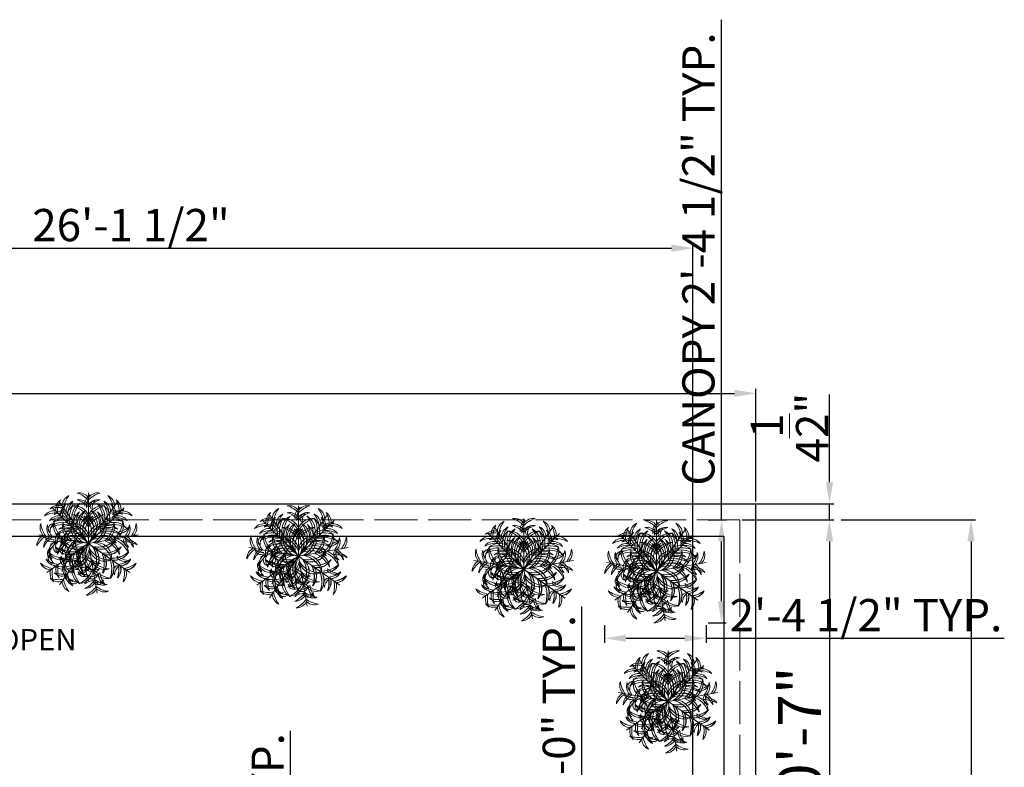
# Model space of a CAD drawing. Units: millimetres. Extents: x 595116 to 630915, y 909473 to 920225.
# Tile 126 of 134: x 629637 to 629912, y 920016 to 920225. Entities that reach past the tile are written whole.
import ezdxf

# ---------------------------------------------------------------- set-up
doc = ezdxf.new("R2010")
doc.units = ezdxf.units.MM
doc.linetypes.add('ACAD_ISO02W100', pattern=[15, 12, -3])
for name, color, linetype, lineweight in [('A-AREA-IDEN', 7, 'Continuous', 20), ('C-PROP', 7, 'Continuous', 25), ('C-PROP-REF', 240, 'ACAD_ISO02W100', 13), ('Dimension', 3, 'Continuous', 18), ('L-PLNT', 85, 'Continuous', 13)]:
    doc.layers.add(name, color=color, linetype=linetype, lineweight=lineweight)
doc.styles.get("Standard").update_dxf_attribs({"font": 'arial.ttf'})
doc.dimstyles.new('ISO-25', dxfattribs={"dimtxt": 9, "dimasz": 6, "dimexe": 1.25, "dimexo": 0.625, "dimtad": 1, "dimlunit": 4, "dimtxsty": 'Standard', "dimcen": 2.5, "dimadec": 0, "dimazin": 0, "dimtfac": 1, "dimtmove": 0, "dimatfit": 3, "dimfxl": 1, "dimarcsym": 0})

# ---------------------------------------------------------------- blocks, each defined once
blk = doc.blocks.new('A$C5D061C3B')
for p, q in [((3.377, 6.679), (3.377, 3.377)), ((1.483, 6.082), (3.377, 3.377)), ((5.259, 6.086), (3.365, 3.381)), ((1.03, 5.716), (3.365, 3.381)), ((5.712, 5.712), (3.377, 3.377)), ((0.125, 3.951), (3.377, 3.377)), ((6.629, 3.951), (3.377, 3.377)), ((0.66, 1.487), (3.365, 3.381)), ((1.483, 0.672), (3.377, 3.377)), ((6.07, 1.487), (3.365, 3.381)), ((3.951, 0.125), (3.377, 3.377)), ((6.082, 1.483), (3.377, 3.377))]:
    blk.add_line(p, q)
for centre, radius, start, end in [((2.419, 5.816), 0.762, 115.37567, 178.71003), ((3.438, 5.44), 1.715, 141.62064, 170.92372), ((2.763, 5.924), 0.762, 36.28997, 99.62433), ((2.145, 5.032), 1.715, 44.07628, 73.37936), ((3.901, 5.939), 0.762, 125.37567, 188.71003), ((4.969, 5.745), 1.715, 151.62064, 180.92372), ((3.991, 5.924), 0.762, 80.37567, 143.71003), ((4.61, 5.032), 1.715, 106.62064, 135.92372), ((3.305, 5.444), 1.715, 9.07628, 38.37936), ((4.323, 5.82), 0.762, 1.28997, 64.62433), ((1.413, 5.111), 0.762, 71.28997, 134.62433), ((1.998, 5.617), 0.762, 125.37567, 188.71003), ((3.066, 5.423), 1.715, 151.62064, 180.92372), ((2.317, 5.298), 0.762, 125.37567, 188.71003), ((3.385, 5.104), 1.715, 151.62064, 180.92372), ((2.678, 5.447), 0.762, 115.37567, 178.71003), ((3.035, 5.062), 1.056, 129.60629, 199.75109), ((3.696, 5.07), 1.715, 141.62064, 170.92372), ((3.894, 4.989), 1.77, 149.96343, 193.62881), ((3.344, 5.089), 1.056, 119.60629, 189.75109), ((2.422, 4.799), 1.056, 25.24891, 95.39371), ((1.866, 4.14), 1.77, 31.37119, 75.03657), ((4.177, 4.869), 1.77, 139.96343, 183.62881), ((2.763, 5.474), 0.762, 36.28997, 99.62433), ((2.145, 4.581), 1.715, 44.07628, 73.37936), ((3.991, 5.474), 0.762, 80.37567, 143.71003), ((4.61, 4.581), 1.715, 106.62064, 135.92372), ((4.332, 4.799), 1.056, 84.60629, 154.75109), ((4.888, 4.14), 1.77, 104.96343, 148.62881), ((3.871, 5.832), 0.38, 94.742, 213.74753), ((4.447, 5.681), 0.826, 139.61802, 183.21064), ((3.398, 5.094), 1.056, 350.24891, 60.39371), ((2.565, 4.873), 1.77, 356.37119, 40.03657), ((2.848, 4.985), 1.77, 346.37119, 30.03657), ((3.707, 5.058), 1.056, 340.24891, 50.39371), ((4.064, 5.451), 0.762, 1.28997, 64.62433), ((3.046, 5.075), 1.715, 9.07628, 38.37936), ((3.357, 5.1), 1.715, 359.07628, 28.37936), ((4.425, 5.294), 0.762, 351.28997, 54.62433), ((4.744, 5.613), 0.762, 351.28997, 54.62433), ((3.676, 5.419), 1.715, 359.07628, 28.37936), ((1.13, 4.748), 0.762, 81.28997, 144.62433), ((1.324, 3.68), 1.715, 89.07628, 118.37936), ((1.448, 4.43), 0.762, 81.28997, 144.62433), ((1.419, 4.026), 1.715, 79.07628, 108.37936), ((1.671, 4.742), 0.762, 71.28997, 134.62433), ((1.677, 3.657), 1.715, 79.07628, 108.37936), ((1.991, 5.462), 0.38, 139.742, 258.74753), ((2.505, 5.763), 0.826, 184.61802, 228.21064), ((2.422, 4.198), 1.056, 25.24891, 95.39371), ((1.866, 3.54), 1.77, 31.37119, 75.03657), ((3.46, 4.637), 1.056, 129.60629, 199.75109), ((4.319, 4.565), 1.77, 149.96343, 193.62881), ((3.688, 4.597), 1.056, 119.60629, 189.75109), ((4.522, 4.377), 1.77, 139.96343, 183.62881), ((3.868, 4.321), 1.029, 121.36542, 221.57406), ((4.556, 4.237), 1.557, 141.81221, 203.33354), ((4.035, 4.215), 1.029, 111.36542, 211.57406), ((2.707, 4.219), 1.029, 328.42594, 68.63458), ((2.044, 4.017), 1.557, 346.66646, 48.18779), ((4.698, 4.013), 1.557, 131.81221, 193.33354), ((4.332, 4.198), 1.056, 84.60629, 154.75109), ((4.888, 3.54), 1.77, 104.96343, 148.62881), ((2.187, 4.233), 1.557, 336.66646, 38.18779), ((2.875, 4.316), 1.029, 318.42594, 58.63458), ((2.221, 4.381), 1.77, 356.37119, 40.03657), ((3.054, 4.602), 1.056, 350.24891, 60.39371), ((3.283, 4.633), 1.056, 340.24891, 50.39371), ((2.424, 4.56), 1.77, 346.37119, 30.03657), ((5.065, 3.661), 1.715, 71.62064, 100.92372), ((5.071, 4.746), 0.762, 45.37567, 108.71003), ((5.564, 4.807), 0.762, 80.37567, 143.71003), ((6.182, 3.914), 1.715, 106.62064, 135.92372), ((5.294, 4.425), 0.762, 35.37567, 98.71003), ((5.419, 3.676), 1.715, 61.62064, 90.92372), ((5.613, 4.744), 0.762, 35.37567, 98.71003), ((0.975, 4.424), 0.762, 160.37567, 223.71003), ((1.962, 4.878), 1.715, 186.62064, 215.92372), ((1.419, 4.346), 0.762, 160.37567, 223.71003), ((2.405, 4.8), 1.715, 186.62064, 215.92372), ((1.12, 4.31), 0.38, 94.742, 213.74753), ((1.642, 3.362), 1.715, 89.07628, 118.37936), ((1.696, 4.159), 0.826, 139.61802, 183.21064), ((1.685, 3.712), 1.056, 70.24891, 140.39371), ((1.757, 2.853), 1.77, 76.37119, 120.03657), ((2.143, 4.564), 1.056, 164.60629, 234.75109), ((1.78, 3.994), 1.056, 60.24891, 130.39371), ((1.702, 3.136), 1.77, 66.37119, 110.03657), ((2.888, 4.998), 1.77, 184.96343, 228.62881), ((2.124, 3.502), 1.056, 60.24891, 130.39371), ((2.734, 4.46), 1.056, 164.60629, 234.75109), ((3.48, 4.893), 1.77, 184.96343, 228.62881), ((2.358, 3.686), 1.029, 3.42594, 103.63458), ((1.93, 3.14), 1.557, 21.66646, 83.18779), ((3.25, 4.435), 1.029, 156.36542, 256.57406), ((3.862, 4.761), 1.557, 176.81221, 238.33354), ((4.397, 3.686), 1.029, 76.36542, 176.57406), ((4.824, 3.14), 1.557, 96.81221, 158.33354), ((2.893, 4.761), 1.557, 301.66646, 3.18779), ((3.504, 4.435), 1.029, 283.42594, 23.63458), ((4.618, 3.506), 1.056, 49.60629, 119.75109), ((5.04, 3.14), 1.77, 69.96343, 113.62881), ((4.963, 3.998), 1.056, 49.60629, 119.75109), ((3.275, 4.893), 1.77, 311.37119, 355.03657), ((4.985, 2.848), 1.77, 59.96343, 103.62881), ((4.02, 4.46), 1.056, 305.24891, 15.39371), ((5.058, 3.707), 1.056, 39.60629, 109.75109), ((3.866, 4.998), 1.77, 311.37119, 355.03657), ((5.1, 3.357), 1.715, 61.62064, 90.92372), ((4.611, 4.564), 1.056, 305.24891, 15.39371), ((4.349, 4.8), 1.715, 324.07628, 353.37936), ((5.335, 4.346), 0.762, 316.28997, 19.62433), ((4.793, 4.878), 1.715, 324.07628, 353.37936), ((5.779, 4.424), 0.762, 316.28997, 19.62433), ((0.762, 3.214), 0.762, 116.28997, 179.62433), ((1.534, 2.451), 1.715, 124.07628, 153.37936), ((1.588, 3.666), 0.38, 94.742, 213.74753), ((2.109, 3.287), 1.056, 70.24891, 140.39371), ((2.182, 2.428), 1.77, 76.37119, 120.03657), ((2.165, 3.515), 0.826, 139.61802, 183.21064), ((2.046, 2.644), 1.77, 66.37119, 110.03657), ((2.426, 2.879), 1.029, 48.42594, 148.63458), ((2.365, 3.045), 1.029, 38.42594, 138.63458), ((2.328, 2.353), 1.557, 56.66646, 118.18779), ((2.387, 3.752), 0.574, 99.98654, 199.40339), ((3.599, 3.314), 1.651, 142.57587, 170.89417), ((2.84, 3.739), 0.372, 69.22575, 210.12788), ((3.109, 3.59), 0.515, 105.43977, 183.66943), ((4.414, 2.358), 1.557, 61.81221, 123.33354), ((4.377, 3.05), 1.029, 41.36542, 141.57406), ((4.316, 2.875), 1.029, 31.36542, 131.57406), ((4.696, 2.648), 1.77, 69.96343, 113.62881), ((4.56, 2.424), 1.77, 59.96343, 103.62881), ((4.633, 3.283), 1.056, 39.60629, 109.75109), ((4.988, 5.812), 1.715, 279.07628, 308.37936), ((5.365, 4.794), 0.762, 271.28997, 334.62433), ((1.206, 3.136), 0.762, 116.28997, 179.62433), ((1.977, 2.373), 1.715, 124.07628, 153.37936), ((1.062, 4.452), 0.826, 229.61802, 273.21064), ((0.91, 3.875), 0.38, 184.742, 303.74753), ((1.811, 2.684), 1.056, 105.24891, 175.39371), ((2.363, 2.022), 1.77, 111.37119, 155.03657), ((2.185, 0.015), 3.567, 70.47721, 111.6585), ((1.447, 3.129), 0.376, 122.05775, 257.85325), ((1.751, 3.126), 0.529, 140.18449, 223.65396), ((2.403, 2.58), 1.056, 105.24891, 175.39371), ((2.955, 1.917), 1.77, 111.37119, 155.03657), ((2.007, 3.071), 0.506, 93.87442, 233.97626), ((2.51, 2.191), 1.557, 66.66646, 128.18779), ((2.729, 4.702), 1.557, 221.81221, 283.33354), ((2.527, 4.039), 1.029, 201.36542, 301.57406), ((4.912, 0.157), 3.567, 115.47721, 156.6585), ((2.489, 2.932), 0.825, 128.75364, 199.09705), ((2.412, 2.943), 0.574, 144.98654, 244.40339), ((2.896, 2.427), 1.029, 83.42594, 183.63458), ((3.359, 1.911), 1.557, 101.66646, 163.18779), ((3.578, 3.49), 1.651, 187.57587, 215.89417), ((2.903, 2.8), 0.855, 116.44767, 194.36723), ((4.744, 1.779), 2.789, 140.40074, 163.13904), ((2.741, 3.253), 0.372, 114.22575, 255.12788), ((3.037, 3.338), 0.515, 150.43977, 228.66943), ((6.727, 2.189), 3.567, 160.47721, 201.6585), ((4.233, 2.187), 1.557, 51.81221, 113.33354), ((4.001, 4.702), 1.557, 256.66646, 318.18779), ((4.013, 4.698), 1.557, 256.66646, 318.18779), ((4.203, 4.039), 1.029, 238.42594, 338.63458), ((4.215, 4.035), 1.029, 238.42594, 338.63458), ((3.395, 1.911), 1.557, 16.81221, 78.33354), ((3.858, 2.427), 1.029, 356.36542, 96.57406), ((3.799, 1.917), 1.77, 24.96343, 68.62881), ((4.352, 2.58), 1.056, 4.60629, 74.75109), ((4.391, 2.022), 1.77, 24.96343, 68.62881), ((4.943, 2.684), 1.056, 4.60629, 74.75109), ((6.053, 3.533), 0.38, 146.25247, 265.258), ((5.741, 1.774), 1.715, 61.62064, 90.92372), ((4.777, 2.373), 1.715, 26.62064, 55.92372), ((6.629, 3.684), 0.826, 176.78936, 220.38198), ((5.935, 2.842), 0.762, 35.37567, 98.71003), ((5.549, 3.136), 0.762, 0.37567, 63.71003), ((1.067, 2.749), 0.376, 122.05775, 257.85325), ((1.873, 4.181), 1.77, 229.96343, 273.62881), ((1.653, 3.348), 1.056, 209.60629, 279.75109), ((1.122, 2.441), 0.38, 139.742, 258.74753), ((1.636, 2.741), 0.826, 184.61802, 228.21064), ((1.37, 2.745), 0.529, 140.18449, 223.65396), ((2.145, 3.693), 1.056, 209.60629, 279.75109), ((2.365, 4.526), 1.77, 229.96343, 273.62881), ((2.328, 4.401), 1.557, 241.81221, 303.33354), ((2.365, 3.709), 1.029, 221.36542, 321.57406), ((3.24, 2.128), 1.056, 150.24891, 220.39371), ((4.099, 2.051), 1.77, 156.37119, 200.03657), ((1.911, 3.359), 1.557, 286.81221, 348.33354), ((2.427, 2.896), 1.029, 266.36542, 6.57406), ((3.45, 2.634), 0.855, 161.44767, 239.36723), ((3.003, 2.844), 0.372, 159.22575, 300.12788), ((3.152, 3.113), 0.515, 195.43977, 273.66943), ((3.697, 2.369), 1.029, 128.42594, 228.63458), ((5.474, 3.214), 2.789, 185.40074, 208.13904), ((4.389, 2.332), 1.557, 146.66646, 208.18779), ((4.035, 2.539), 1.029, 148.42594, 248.63458), ((4.698, 2.741), 1.557, 166.66646, 228.18779), ((4.963, 4.749), 2.789, 230.40074, 253.13904), ((4.435, 3.25), 1.029, 193.42594, 293.63458), ((4.761, 3.862), 1.557, 211.66646, 273.18779), ((2.341, 2.332), 1.557, 331.81221, 33.33354), ((2.353, 2.328), 1.557, 331.81221, 33.33354), ((3.033, 2.369), 1.029, 311.36542, 51.57406), ((3.045, 2.365), 1.029, 311.36542, 51.57406), ((4.365, 4.526), 1.77, 266.37119, 310.03657), ((2.632, 2.051), 1.77, 339.96343, 23.62881), ((4.377, 4.522), 1.77, 266.37119, 310.03657), ((2.644, 2.046), 1.77, 339.96343, 23.62881), ((3.49, 2.128), 1.056, 319.60629, 29.75109), ((3.502, 2.124), 1.056, 319.60629, 29.75109), ((4.585, 3.693), 1.056, 260.24891, 330.39371), ((4.597, 3.688), 1.056, 260.24891, 330.39371), ((4.857, 4.181), 1.77, 266.37119, 310.03657), ((4.869, 4.177), 1.77, 266.37119, 310.03657), ((5.077, 3.348), 1.056, 260.24891, 330.39371), ((5.089, 3.344), 1.056, 260.24891, 330.39371), ((0.926, 2.424), 0.762, 205.37567, 268.71003), ((1.303, 3.442), 1.715, 231.62064, 260.92372), ((1.672, 3.7), 1.715, 231.62064, 260.92372), ((1.295, 2.682), 0.762, 205.37567, 268.71003), ((1.702, 3.619), 1.77, 249.96343, 293.62881), ((1.78, 2.76), 1.056, 229.60629, 299.75109), ((3.086, 1.681), 1.715, 169.07628, 198.37936), ((2.046, 4.111), 1.77, 249.96343, 293.62881), ((2.124, 3.252), 1.056, 229.60629, 299.75109), ((1.908, 2.317), 0.38, 139.742, 258.74753), ((2.422, 2.617), 0.826, 184.61802, 228.21064), ((2.748, 1.784), 1.056, 150.24891, 220.39371), ((3.607, 1.706), 1.77, 156.37119, 200.03657), ((2.405, 2.049), 0.529, 185.18449, 268.65396), ((2.624, 2.192), 0.506, 138.87442, 278.97626), ((3.064, 2.435), 0.825, 173.75364, 244.09705), ((4.177, 1.886), 1.77, 176.37119, 220.03657), ((3.428, 3.603), 1.651, 232.57587, 260.89417), ((2.99, 2.391), 0.574, 189.98654, 289.40339), ((3.688, 2.157), 1.056, 170.24891, 240.39371), ((1.917, 2.955), 1.77, 294.96343, 338.62881), ((2.58, 2.403), 1.056, 274.60629, 344.75109), ((4.522, 2.378), 1.77, 176.37119, 220.03657), ((3.81, 2.493), 0.825, 218.75364, 289.09705), ((3.671, 2.011), 0.506, 183.87442, 323.97626), ((3.942, 2.908), 0.855, 206.44767, 284.36723), ((4.893, 3.48), 1.77, 221.37119, 265.03657), ((4.46, 2.734), 1.056, 215.24891, 285.39371), ((3.124, 1.706), 1.77, 339.96343, 23.62881), ((3.136, 1.702), 1.77, 339.96343, 23.62881), ((3.982, 1.784), 1.056, 319.60629, 29.75109), ((3.994, 1.78), 1.056, 319.60629, 29.75109), ((5.385, 1.584), 0.38, 101.25247, 220.258), ((6.244, 3.948), 1.715, 234.07628, 263.37936), ((5.79, 2.962), 0.762, 226.28997, 289.62433), ((3.645, 1.681), 1.715, 341.62064, 10.92372), ((3.657, 1.677), 1.715, 341.62064, 10.92372), ((5.058, 3.7), 1.715, 279.07628, 308.37936), ((5.07, 3.696), 1.715, 279.07628, 308.37936), ((5.435, 2.682), 0.762, 271.28997, 334.62433), ((5.447, 2.678), 0.762, 271.28997, 334.62433), ((5.427, 3.442), 1.715, 279.07628, 308.37936), ((5.44, 3.438), 1.715, 279.07628, 308.37936), ((5.804, 2.424), 0.762, 271.28997, 334.62433), ((5.816, 2.419), 0.762, 271.28997, 334.62433), ((1.631, 1.417), 0.762, 161.28997, 224.62433), ((2.717, 1.423), 1.715, 169.07628, 198.37936), ((1.671, 2.012), 0.762, 225.37567, 288.71003), ((1.677, 3.098), 1.715, 251.62064, 280.92372), ((2, 1.676), 0.762, 161.28997, 224.62433), ((2.188, 1.837), 0.376, 167.05775, 302.85325), ((2.188, 1.299), 0.376, 167.05775, 302.85325), ((2.405, 1.511), 0.529, 185.18449, 268.65396), ((2.678, 1.307), 0.762, 181.28997, 244.62433), ((3.696, 1.684), 1.715, 189.07628, 218.37936), ((3.344, 1.665), 1.056, 170.24891, 240.39371), ((3.227, 2.169), 0.826, 229.61802, 273.21064), ((3.076, 1.593), 0.38, 184.742, 303.74753), ((2.022, 2.363), 1.77, 294.96343, 338.62881), ((2.684, 1.811), 1.056, 274.60629, 344.75109), ((3.616, 1.755), 0.529, 230.18449, 313.65396), ((3.613, 1.452), 0.376, 212.05775, 347.85325), ((4.998, 2.888), 1.77, 221.37119, 265.03657), ((4.564, 2.143), 1.056, 215.24891, 285.39371), ((4.79, 1.377), 0.762, 181.28997, 244.62433), ((5.808, 1.754), 1.715, 189.07628, 218.37936), ((5.899, 1.283), 0.826, 131.78936, 175.38198), ((4.73, 1.676), 0.762, 315.37567, 18.71003), ((4.742, 1.671), 0.762, 315.37567, 18.71003), ((4.014, 1.423), 1.715, 341.62064, 10.92372), ((5.099, 1.417), 0.762, 315.37567, 18.71003), ((1.419, 2.729), 1.715, 251.62064, 280.92372), ((1.413, 1.643), 0.762, 225.37567, 288.71003), ((2.419, 0.938), 0.762, 181.28997, 244.62433), ((3.438, 1.315), 1.715, 189.07628, 218.37936), ((2.583, 1.701), 0.826, 229.61802, 273.21064), ((2.432, 1.124), 0.38, 184.742, 303.74753), ((2.373, 1.977), 1.715, 296.62064, 325.92372), ((3.136, 1.206), 0.762, 270.37567, 333.71003), ((3.68, 0.113), 0.826, 86.78936, 130.38198), ((3.528, 0.69), 0.38, 56.25247, 175.258), ((3.997, 1.374), 0.529, 230.18449, 313.65396), ((3.994, 1.071), 0.376, 212.05775, 347.85325), ((4.8, 2.405), 1.715, 234.07628, 263.37936), ((4.346, 1.419), 0.762, 226.28997, 289.62433), ((2.451, 1.534), 1.715, 296.62064, 325.92372), ((3.214, 0.762), 0.762, 270.37567, 333.71003), ((4.878, 1.962), 1.715, 234.07628, 263.37936), ((4.424, 0.975), 0.762, 226.28997, 289.62433)]:
    blk.add_arc(centre, radius, start, end)
blk = doc.blocks.new('*D121')
at = {"layer": 'Defpoints', "color": 0, "transparency": 16777216}
for p in [(629838.04, 920084.93), (629838.04, 919957.93), (629863.03, 919957.93)]:
    blk.add_point(p, dxfattribs=at)
at = {"layer": 'Dimension', "color": 0, "lineweight": -2, "transparency": 16777216}
for p, q in [((629838.67, 920084.93), (629864.28, 920084.93)), ((629863.03, 920078.93), (629863.03, 919963.93)), ((629838.67, 919957.93), (629864.28, 919957.93))]:
    blk.add_line(p, q, dxfattribs=at)
at = {"layer": 'Dimension', "color": 0, "transparency": 16777216}
for points in [[(629862.03, 920078.93), (629864.03, 920078.93), (629863.03, 920084.93)], [(629862.03, 919963.93), (629864.03, 919963.93), (629863.03, 919957.93)]]:
    blk.add_solid(points, dxfattribs=at)
at = {"layer": 'Dimension', "color": 0, "transparency": 16777216, "insert": (629856.28, 920021.43), "char_height": 12, "attachment_point": 5, "rotation": 90}
blk.add_mtext('10\'-7"', dxfattribs=at)
blk = doc.blocks.new('*D124')
at = {"layer": 'Defpoints', "color": 0, "transparency": 16777216}
for p in [(629865.75, 920084.93), (629865.75, 919141.93), (629902.57, 919141.93)]:
    blk.add_point(p, dxfattribs=at)
at = {"layer": 'Dimension', "color": 0, "lineweight": -2, "transparency": 16777216}
for p, q in [((629866.37, 920084.93), (629903.82, 920084.93)), ((629902.57, 920078.93), (629902.57, 919147.93)), ((629866.37, 919141.93), (629903.82, 919141.93))]:
    blk.add_line(p, q, dxfattribs=at)
at = {"layer": 'Dimension', "color": 0, "transparency": 16777216}
for points in [[(629901.57, 920078.93), (629903.57, 920078.93), (629902.57, 920084.93)], [(629901.57, 919147.93), (629903.57, 919147.93), (629902.57, 919141.93)]]:
    blk.add_solid(points, dxfattribs=at)
at = {"layer": 'Dimension', "color": 0, "transparency": 16777216, "insert": (629897.35, 919613.43), "char_height": 9, "attachment_point": 5, "rotation": 90}
blk.add_mtext('78\'-7"', dxfattribs=at)
blk = doc.blocks.new('*D125')
at = {"layer": 'Defpoints', "color": 0, "transparency": 16777216}
for p in [(629842.54, 920120.25), (629311.54, 920089.43), (629842.54, 920089.43)]:
    blk.add_point(p, dxfattribs=at)
at = {"layer": 'Dimension', "color": 0, "lineweight": -2, "transparency": 16777216}
for p, q in [((629311.54, 920090.05), (629311.54, 920121.5)), ((629317.54, 920120.25), (629836.54, 920120.25)), ((629842.54, 920090.05), (629842.54, 920121.5))]:
    blk.add_line(p, q, dxfattribs=at)
at = {"layer": 'Dimension', "color": 0, "transparency": 16777216}
for points in [[(629317.54, 920121.25), (629317.54, 920119.25), (629311.54, 920120.25)], [(629836.54, 920121.25), (629836.54, 920119.25), (629842.54, 920120.25)]]:
    blk.add_solid(points, dxfattribs=at)
at = {"layer": 'Dimension', "color": 0, "transparency": 16777216, "insert": (629577.04, 920125.47), "char_height": 9, "attachment_point": 5}
blk.add_mtext('44\'-3"', dxfattribs=at)
blk = doc.blocks.new('*D126')
at = {"layer": 'Defpoints', "color": 0, "transparency": 16777216}
for p in [(629838.04, 920089.43), (629863.07, 920089.43), (629838.04, 920084.93)]:
    blk.add_point(p, dxfattribs=at)
at = {"layer": 'Dimension', "color": 0, "lineweight": -2, "transparency": 16777216}
for p, q in [((629863.07, 920095.43), (629863.07, 920119.95)), ((629838.67, 920089.43), (629864.32, 920089.43)), ((629863.07, 920084.93), (629863.07, 920089.43)), ((629838.67, 920084.93), (629864.32, 920084.93)), ((629863.07, 920078.93), (629863.07, 920072.93))]:
    blk.add_line(p, q, dxfattribs=at)
at = {"layer": 'Dimension', "color": 0, "transparency": 16777216}
for points in [[(629862.07, 920095.43), (629864.07, 920095.43), (629863.07, 920089.43)], [(629862.07, 920078.93), (629864.07, 920078.93), (629863.07, 920084.93)]]:
    blk.add_solid(points, dxfattribs=at)
at = {"layer": 'Dimension', "color": 0, "transparency": 16777216, "insert": (629851.91, 920110.69), "char_height": 9, "attachment_point": 5, "rotation": 90}
blk.add_mtext('4{\\H1x;\\S1/2;}"', dxfattribs=at)
blk = doc.blocks.new('*D160')
at = {"layer": 'Defpoints', "color": 0, "transparency": 16777216}
for p in [(629788.54, 919957.93), (629793.96, 919957.93), (629788.54, 919921.79)]:
    blk.add_point(p, dxfattribs=at)
at = {"layer": 'Dimension', "color": 0, "lineweight": -2, "transparency": 16777216}
for p, q in [((629793.96, 919957.93), (629793.96, 920060.8)), ((629789.17, 919957.93), (629795.21, 919957.93)), ((629793.96, 919927.79), (629793.96, 919951.93)), ((629789.17, 919921.79), (629795.21, 919921.79))]:
    blk.add_line(p, q, dxfattribs=at)
at = {"layer": 'Dimension', "color": 0, "transparency": 16777216}
for points in [[(629792.96, 919951.93), (629794.96, 919951.93), (629793.96, 919957.93)], [(629792.96, 919927.79), (629794.96, 919927.79), (629793.96, 919921.79)]]:
    blk.add_solid(points, dxfattribs=at)
at = {"layer": 'Dimension', "color": 0, "transparency": 16777216, "insert": (629788.68, 920012.36), "char_height": 9, "attachment_point": 5, "rotation": 90}
blk.add_mtext('DOOR 3\'-0" TYP.', dxfattribs=at)
blk = doc.blocks.new('*D197')
at = {"layer": 'Defpoints', "color": 0, "transparency": 16777216}
for p in [(629709.04, 919957.93), (629712.64, 919957.93), (629709.04, 919948.93)]:
    blk.add_point(p, dxfattribs=at)
at = {"layer": 'Dimension', "color": 0, "lineweight": -2, "transparency": 16777216}
for p, q in [((629712.64, 919963.93), (629712.64, 920026.04)), ((629709.67, 919957.93), (629713.89, 919957.93)), ((629712.64, 919948.93), (629712.64, 919957.93)), ((629709.67, 919948.93), (629713.89, 919948.93)), ((629712.64, 919942.93), (629712.64, 919936.93))]:
    blk.add_line(p, q, dxfattribs=at)
at = {"layer": 'Dimension', "color": 0, "transparency": 16777216}
for points in [[(629711.64, 919963.93), (629713.64, 919963.93), (629712.64, 919957.93)], [(629711.64, 919942.93), (629713.64, 919942.93), (629712.64, 919948.93)]]:
    blk.add_solid(points, dxfattribs=at)
at = {"layer": 'Dimension', "color": 0, "transparency": 16777216, "insert": (629707.42, 919997.98), "char_height": 9, "attachment_point": 5, "rotation": 90}
blk.add_mtext('0\'-9" TYP.', dxfattribs=at)
blk = doc.blocks.new('*D212')
at = {"layer": 'Defpoints', "color": 0, "transparency": 16777216}
for p in [(629828.63, 920084.93), (629832.94, 920084.93), (629828.63, 920056.22)]:
    blk.add_point(p, dxfattribs=at)
at = {"layer": 'Dimension', "color": 0, "lineweight": -2, "transparency": 16777216}
for p, q in [((629832.94, 920084.93), (629832.94, 920224.5)), ((629829.25, 920084.93), (629834.19, 920084.93)), ((629832.94, 920062.22), (629832.94, 920078.93)), ((629829.25, 920056.22), (629834.19, 920056.22))]:
    blk.add_line(p, q, dxfattribs=at)
at = {"layer": 'Dimension', "color": 0, "transparency": 16777216}
for points in [[(629831.94, 920078.93), (629833.94, 920078.93), (629832.94, 920084.93)], [(629831.94, 920062.22), (629833.94, 920062.22), (629832.94, 920056.22)]]:
    blk.add_solid(points, dxfattribs=at)
at = {"layer": 'Dimension', "color": 0, "transparency": 16777216, "insert": (629827.65, 920157.72), "char_height": 9, "attachment_point": 5, "rotation": 90}
blk.add_mtext('CANOPY 2\'-4 1/2" TYP.', dxfattribs=at)
blk = doc.blocks.new('*D213')
at = {"layer": 'Defpoints', "color": 0, "transparency": 16777216}
for p in [(629800.31, 920056.22), (629828.63, 920056.22), (629828.63, 920051.91)]:
    blk.add_point(p, dxfattribs=at)
at = {"layer": 'Dimension', "color": 0, "lineweight": -2, "transparency": 16777216}
for p, q in [((629800.31, 920055.59), (629800.31, 920050.66)), ((629828.63, 920055.59), (629828.63, 920050.66)), ((629806.31, 920051.91), (629822.63, 920051.91)), ((629828.63, 920051.91), (629911.86, 920051.91))]:
    blk.add_line(p, q, dxfattribs=at)
at = {"layer": 'Dimension', "color": 0, "transparency": 16777216}
for points in [[(629806.31, 920052.91), (629806.31, 920050.91), (629800.31, 920051.91)], [(629822.63, 920052.91), (629822.63, 920050.91), (629828.63, 920051.91)]]:
    blk.add_solid(points, dxfattribs=at)
at = {"layer": 'Dimension', "color": 0, "transparency": 16777216, "insert": (629873.25, 920057.19), "char_height": 9, "attachment_point": 5}
blk.add_mtext('2\'-4 1/2" TYP.', dxfattribs=at)
blk = doc.blocks.new('*D220')
at = {"layer": 'Defpoints', "color": 0, "transparency": 16777216}
for p in [(629824.95, 920160.76), (629511.27, 919302.01), (629824.95, 919302.01)]:
    blk.add_point(p, dxfattribs=at)
at = {"layer": 'Dimension', "color": 0, "lineweight": -2, "transparency": 16777216}
for p, q in [((629511.27, 919302.63), (629511.27, 920162.01)), ((629517.27, 920160.76), (629818.95, 920160.76)), ((629824.95, 919302.63), (629824.95, 920162.01))]:
    blk.add_line(p, q, dxfattribs=at)
at = {"layer": 'Dimension', "color": 0, "transparency": 16777216}
for points in [[(629517.27, 920161.76), (629517.27, 920159.76), (629511.27, 920160.76)], [(629818.95, 920161.76), (629818.95, 920159.76), (629824.95, 920160.76)]]:
    blk.add_solid(points, dxfattribs=at)
at = {"layer": 'Dimension', "color": 0, "transparency": 16777216, "insert": (629668.11, 920166.03), "char_height": 9, "attachment_point": 5}
blk.add_mtext('26\'-1 1/2"', dxfattribs=at)

msp = doc.modelspace()

# ---------------------------------------------------------------- linework, layer by layer
at = {"layer": 'C-PROP'}
for p, q in [((629842.541, 919957.928), (629842.541, 920089.428)), ((629320.541, 920080.428), (629833.541, 920080.428)), ((629833.541, 920080.428), (629833.541, 919957.928))]:
    msp.add_line(p, q, dxfattribs=at)
msp.add_lwpolyline([(629311.541, 920089.428), (629842.541, 920089.428)], dxfattribs=at)
at = {"layer": 'C-PROP-REF'}
for p, q in [((629316.041, 920084.928), (629838.041, 920084.928)), ((629838.041, 920084.928), (629838.041, 919141.928))]:
    msp.add_line(p, q, dxfattribs=at)

# ---------------------------------------------------------------- block references
at = {"layer": 'L-PLNT', "xscale": 4.271269117679152, "yscale": 4.271269117679152, "zscale": 4.271269117679152}
for p in [(629641.813, 920063.917), (629700.448, 920060.36), (629763.308, 920056.777), (629800.314, 920056.216), (629803.597, 920019.89)]:
    msp.add_blockref('A$C5D061C3B', p, dxfattribs=at)

# ---------------------------------------------------------------- texts
at = {"layer": 'A-AREA-IDEN', "insert": (629589.324, 920054.511), "char_height": 6, "attachment_point": 1}
msp.add_mtext_dynamic_manual_height_columns('{REAR SIDE OPEN\\P       AREA}', width=127.44285, gutter_width=12.5, heights=[0], dxfattribs=at)

# ---------------------------------------------------------------- dimensions: what is measured, and where the dimension line sits
at = {"layer": 'Dimension'}
for base, p1, p2, text, picture, middle in [((629832.936, 920084.935), (629828.628, 920056.216), (629828.628, 920084.935), 'CANOPY <> TYP.', '*D212', (629827.654, 920157.719)), ((629793.962, 919957.928), (629788.541, 919921.789), (629788.541, 919957.928), 'DOOR <> TYP.', '*D160', (629788.677, 920012.364)), ((629712.641, 919957.928), (629709.041, 919948.928), (629709.041, 919957.928), '<> TYP.', '*D197', (629707.421, 919997.982))]:
    dim = msp.add_linear_dim(base=base, p1=p1, p2=p2, angle=90, text=text, dimstyle='ISO-25', override={"dimdec": 1, "dimlfac": 1, "dimrnd": 0, "dimzin": 1, "dimdsep": 46, "dimlunit": 4, "dimfrac": 2}, dxfattribs=at)
    dim.commit()
    dim.dimension.update_dxf_attribs({"geometry": picture, "text_midpoint": middle})
for base, p1, p2, override, picture, middle in [((629824.951, 920160.756), (629511.274, 919302.009), (629824.951, 919302.009), {"dimdec": 1, "dimlfac": 1, "dimrnd": 0, "dimzin": 1, "dimdsep": 46, "dimlunit": 4, "dimfrac": 2}, '*D220', (629668.113, 920166.035)), ((629842.541, 920120.249), (629311.541, 920089.428), (629842.541, 920089.428), {"dimclrd": 0, "dimclre": 0, "dimclrt": 0}, '*D125', (629577.041, 920125.472))]:
    dim = msp.add_linear_dim(base=base, p1=p1, p2=p2, dimstyle='ISO-25', override=override, dxfattribs=at)
    dim.commit()
    dim.dimension.update_dxf_attribs({"geometry": picture, "text_midpoint": middle})
for base, p1, p2, override, picture, middle in [((629863.073, 920089.428), (629838.041, 920084.928), (629838.041, 920089.428), {"dimclrd": 0, "dimclre": 0, "dimclrt": 0}, '*D126', (629851.911, 920110.687)), ((629863.031, 919957.928), (629838.041, 920084.928), (629838.041, 919957.928), {"dimtxt": 12, "dimclrd": 0, "dimclre": 0, "dimclrt": 0}, '*D121', (629856.279, 920021.428)), ((629902.574, 919141.928), (629865.746, 920084.928), (629865.746, 919141.928), {"dimclrd": 0, "dimclre": 0, "dimclrt": 0}, '*D124', (629897.354, 919613.428))]:
    dim = msp.add_linear_dim(base=base, p1=p1, p2=p2, angle=90, dimstyle='ISO-25', override=override, dxfattribs=at)
    dim.commit()
    dim.dimension.update_dxf_attribs({"geometry": picture, "text_midpoint": middle})
dim = msp.add_linear_dim(base=(629828.628, 920051.908), p1=(629800.314, 920056.216), p2=(629828.628, 920056.216), text='<> TYP.', dimstyle='ISO-25', override={"dimdec": 1, "dimlfac": 1, "dimrnd": 0, "dimzin": 1, "dimdsep": 46, "dimlunit": 4, "dimfrac": 2}, dxfattribs=at)
dim.commit()
dim.dimension.update_dxf_attribs({"geometry": '*D213', "text_midpoint": (629873.245, 920057.186)})

doc.saveas('drawing.dxf')
